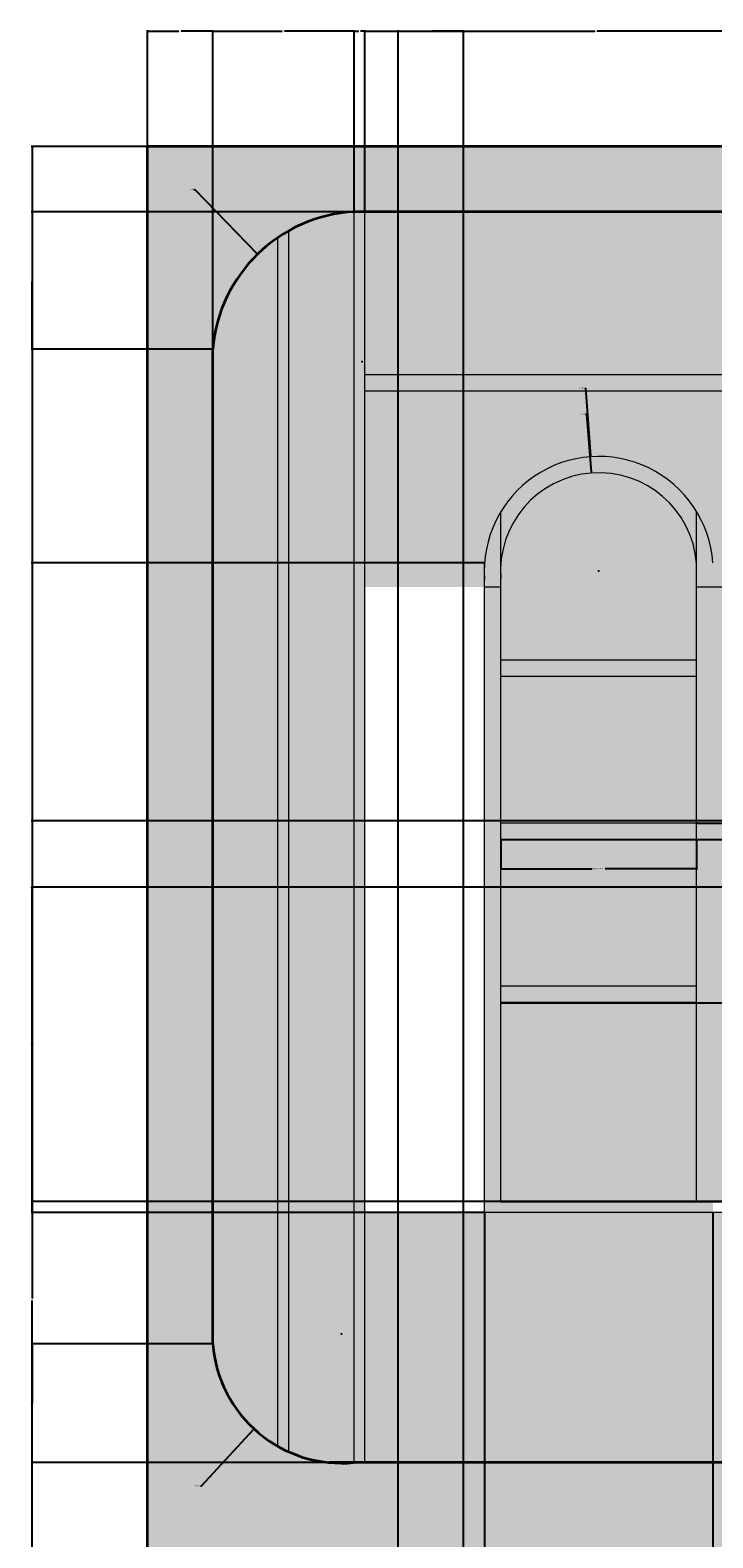
# Model space of a CAD drawing. Units: inches. Extents: x 2051 to 2334, y 814 to 1281.
# Tile 3 of 4: x 2051 to 2177, y 1003 to 1281. Entities that reach past the tile are written whole.
import ezdxf

# ---------------------------------------------------------------- set-up
doc = ezdxf.new("R2010")
doc.units = ezdxf.units.IN
for name, color, linetype, lineweight in [('A-ANNO-DIMS', 2, 'Continuous', 18), ('A-ELEV-FRAM', 7, 'Continuous', 35), ('A-ELEV-TRIM', 7, 'Continuous', 18), ('A-ELEV-TRIM-PATT', 7, 'Continuous', 13), ('A-GLAZ', 4, 'Continuous', 18), ('A-GLAZ-PATT', 4, 'Continuous', 13), ('A-ROOF', 7, 'Continuous', 35)]:
    doc.layers.add(name, color=color, linetype=linetype, lineweight=lineweight)
doc.layers.add('A-ELEV-FRAM-PATT', color=251, linetype='Continuous', lineweight=13, true_color=0x636466)
doc.layers.add('A-WALL-PATT', color=9, linetype='Continuous', lineweight=13, true_color=0xc7c8ca)
doc.styles.get("Standard").update_dxf_attribs({"font": 'arial.ttf'})
doc.dimstyles.get("Standard").update_dxf_attribs({"dimtxt": 0.18, "dimasz": 0.18, "dimexe": 0.18, "dimexo": 0.0625, "dimgap": 0.09, "dimtad": 0, "dimtih": 1, "dimtoh": 1, "dimdec": 4, "dimzin": 0, "dimdsep": 46, "dimtxsty": 'Standard', "dimcen": 0.09, "dimadec": 0, "dimazin": 0, "dimtfac": 1, "dimtdec": 4, "dimtofl": 0, "dimtmove": 0, "dimatfit": 3, "dimfxl": 1, "dimtolj": 1, "dimtzin": 0, "dimarcsym": 0})

# ---------------------------------------------------------------- blocks, each defined once
blk = doc.blocks.new('ARCH-LIGHT-TRANSOM-36X3')
for p, q in [((36, 3), (0, 3)), ((36, 0), (0, 0))]:
    blk.add_line(p, q)
blk = doc.blocks.new('*D5')
at = {"layer": 'A-ANNO-DIMS', "color": 0, "lineweight": -2, "transparency": 16777216}
for p, q in [((2137.93, 1131.75), (2137.93, 1126.23)), ((2173.93, 1131.75), (2173.93, 1126.23)), ((2138.11, 1126.41), (2154.73, 1126.41)), ((2173.75, 1126.41), (2157.12, 1126.41))]:
    blk.add_line(p, q, dxfattribs=at)
at = {"layer": 'A-ANNO-DIMS', "color": 0, "transparency": 16777216}
for points in [[(2138.11, 1126.44), (2138.11, 1126.38), (2137.93, 1126.41)], [(2173.75, 1126.44), (2173.75, 1126.38), (2173.93, 1126.41)]]:
    blk.add_solid(points, dxfattribs=at)
at = {"layer": 'Defpoints', "color": 0, "transparency": 16777216}
for p in [(2137.93, 1131.81), (2173.93, 1131.81), (2173.93, 1126.41)]:
    blk.add_point(p, dxfattribs=at)
at = {"layer": 'A-ANNO-DIMS', "color": 0, "transparency": 16777216, "insert": (2155.93, 1126.41), "char_height": 0.18, "attachment_point": 5}
blk.add_mtext('\\A1;TRANSOM 36 TYP.', dxfattribs=at)
blk = doc.blocks.new('*D6')
at = {"layer": 'A-ANNO-DIMS', "color": 0, "lineweight": -2, "transparency": 16777216}
for p, q in [((2173.99, 1134.81), (2179.51, 1134.81)), ((2179.33, 1134.63), (2179.33, 1133.5)), ((2173.99, 1131.81), (2179.51, 1131.81)), ((2179.33, 1131.99), (2179.33, 1133.13))]:
    blk.add_line(p, q, dxfattribs=at)
at = {"layer": 'A-ANNO-DIMS', "color": 0, "transparency": 16777216}
for points in [[(2179.3, 1134.63), (2179.36, 1134.63), (2179.33, 1134.81)], [(2179.3, 1131.99), (2179.36, 1131.99), (2179.33, 1131.81)]]:
    blk.add_solid(points, dxfattribs=at)
at = {"layer": 'Defpoints', "color": 0, "transparency": 16777216}
for p in [(2173.93, 1134.81), (2179.33, 1134.81), (2173.93, 1131.81)]:
    blk.add_point(p, dxfattribs=at)
at = {"layer": 'A-ANNO-DIMS', "color": 0, "transparency": 16777216, "insert": (2179.33, 1133.31), "char_height": 0.18, "attachment_point": 5}
blk.add_mtext('\\A1;3 TYP.', dxfattribs=at)
blk = doc.blocks.new('*D8')
at = {"layer": 'A-ANNO-DIMS', "color": 0, "lineweight": -2, "transparency": 16777216}
for p, q in [((2072.87, 1259.24), (2051.53, 1259.24)), ((2051.71, 1259.06), (2051.71, 1047.42)), ((2051.71, 835.42), (2051.71, 1047.06)), ((2072.87, 835.24), (2051.53, 835.24))]:
    blk.add_line(p, q, dxfattribs=at)
at = {"layer": 'A-ANNO-DIMS', "color": 0, "transparency": 16777216}
for points in [[(2051.68, 1259.06), (2051.74, 1259.06), (2051.71, 1259.24)], [(2051.68, 835.42), (2051.74, 835.42), (2051.71, 835.24)]]:
    blk.add_solid(points, dxfattribs=at)
at = {"layer": 'Defpoints', "color": 0, "transparency": 16777216}
for p in [(2051.71, 1259.24), (2072.93, 1259.24), (2072.93, 835.24)]:
    blk.add_point(p, dxfattribs=at)
at = {"layer": 'A-ANNO-DIMS', "color": 0, "transparency": 16777216, "insert": (2051.71, 1047.24), "char_height": 0.18, "attachment_point": 5}
blk.add_mtext('\\A1;424', dxfattribs=at)
blk = doc.blocks.new('*D16')
at = {"layer": 'A-ANNO-DIMS', "color": 0, "lineweight": -2, "transparency": 16777216}
for p, q in [((2072.93, 1259.31), (2072.93, 1280.64)), ((2073.11, 1280.46), (2078.72, 1280.46)), ((2084.75, 1280.46), (2079.14, 1280.46)), ((2084.93, 1222.02), (2084.93, 1280.64))]:
    blk.add_line(p, q, dxfattribs=at)
at = {"layer": 'A-ANNO-DIMS', "color": 0, "transparency": 16777216}
for points in [[(2073.11, 1280.49), (2073.11, 1280.43), (2072.93, 1280.46)], [(2084.75, 1280.49), (2084.75, 1280.43), (2084.93, 1280.46)]]:
    blk.add_solid(points, dxfattribs=at)
at = {"layer": 'Defpoints', "color": 0, "transparency": 16777216}
for p in [(2084.93, 1280.46), (2072.93, 1259.24), (2084.93, 1221.95)]:
    blk.add_point(p, dxfattribs=at)
at = {"layer": 'A-ANNO-DIMS', "color": 0, "transparency": 16777216, "insert": (2078.93, 1280.46), "char_height": 0.18, "attachment_point": 5}
blk.add_mtext('\\A1;12', dxfattribs=at)
blk = doc.blocks.new('*D17')
at = {"layer": 'A-ANNO-DIMS', "color": 0, "lineweight": -2, "transparency": 16777216}
for p, q in [((2084.93, 1222.02), (2084.93, 1280.64)), ((2085.11, 1280.46), (2097.71, 1280.46)), ((2110.75, 1280.46), (2098.15, 1280.46)), ((2110.93, 1247.31), (2110.93, 1280.64))]:
    blk.add_line(p, q, dxfattribs=at)
at = {"layer": 'A-ANNO-DIMS', "color": 0, "transparency": 16777216}
for points in [[(2085.11, 1280.49), (2085.11, 1280.43), (2084.93, 1280.46)], [(2110.75, 1280.49), (2110.75, 1280.43), (2110.93, 1280.46)]]:
    blk.add_solid(points, dxfattribs=at)
at = {"layer": 'Defpoints', "color": 0, "transparency": 16777216}
for p in [(2110.93, 1280.46), (2110.93, 1247.24), (2084.93, 1221.95)]:
    blk.add_point(p, dxfattribs=at)
at = {"layer": 'A-ANNO-DIMS', "color": 0, "transparency": 16777216, "insert": (2097.93, 1280.46), "char_height": 0.18, "attachment_point": 5}
blk.add_mtext('\\A1;26', dxfattribs=at)
blk = doc.blocks.new('*D18')
at = {"layer": 'A-ANNO-DIMS', "color": 0, "lineweight": -2, "transparency": 16777216}
for p, q in [((2110.93, 1247.31), (2110.93, 1280.64)), ((2111.11, 1280.46), (2111.78, 1280.46)), ((2112.75, 1280.46), (2112.08, 1280.46)), ((2112.93, 1247.31), (2112.93, 1280.64))]:
    blk.add_line(p, q, dxfattribs=at)
at = {"layer": 'A-ANNO-DIMS', "color": 0, "transparency": 16777216}
for points in [[(2111.11, 1280.49), (2111.11, 1280.43), (2110.93, 1280.46)], [(2112.75, 1280.49), (2112.75, 1280.43), (2112.93, 1280.46)]]:
    blk.add_solid(points, dxfattribs=at)
at = {"layer": 'Defpoints', "color": 0, "transparency": 16777216}
for p in [(2112.93, 1280.46), (2110.93, 1247.24), (2112.93, 1247.24)]:
    blk.add_point(p, dxfattribs=at)
at = {"layer": 'A-ANNO-DIMS', "color": 0, "transparency": 16777216, "insert": (2111.93, 1280.46), "char_height": 0.18, "attachment_point": 5}
blk.add_mtext('\\A1;2', dxfattribs=at)
blk = doc.blocks.new('*D19')
at = {"layer": 'A-ANNO-DIMS', "color": 0, "lineweight": -2, "transparency": 16777216}
for p, q in [((2112.93, 1247.31), (2112.93, 1280.64)), ((2113.11, 1280.46), (2155.21, 1280.46)), ((2197.75, 1280.46), (2155.65, 1280.46)), ((2197.93, 1247.31), (2197.93, 1280.64))]:
    blk.add_line(p, q, dxfattribs=at)
at = {"layer": 'A-ANNO-DIMS', "color": 0, "transparency": 16777216}
for points in [[(2113.11, 1280.49), (2113.11, 1280.43), (2112.93, 1280.46)], [(2197.75, 1280.49), (2197.75, 1280.43), (2197.93, 1280.46)]]:
    blk.add_solid(points, dxfattribs=at)
at = {"layer": 'Defpoints', "color": 0, "transparency": 16777216}
for p in [(2197.93, 1280.46), (2112.93, 1247.24), (2197.93, 1247.24)]:
    blk.add_point(p, dxfattribs=at)
at = {"layer": 'A-ANNO-DIMS', "color": 0, "transparency": 16777216, "insert": (2155.43, 1280.46), "char_height": 0.18, "attachment_point": 5}
blk.add_mtext('\\A1;85', dxfattribs=at)
blk = doc.blocks.new('*D23')
at = {"layer": 'A-ANNO-DIMS', "color": 0, "lineweight": -2, "transparency": 16777216}
for p, q in [((2084.87, 1039.06), (2051.53, 1039.06)), ((2051.71, 1038.88), (2051.71, 1028.33)), ((2051.71, 1017.42), (2051.71, 1027.97)), ((2110.87, 1017.24), (2051.53, 1017.24))]:
    blk.add_line(p, q, dxfattribs=at)
at = {"layer": 'A-ANNO-DIMS', "color": 0, "transparency": 16777216}
for points in [[(2051.68, 1038.88), (2051.74, 1038.88), (2051.71, 1039.06)], [(2051.68, 1017.42), (2051.74, 1017.42), (2051.71, 1017.24)]]:
    blk.add_solid(points, dxfattribs=at)
at = {"layer": 'Defpoints', "color": 0, "transparency": 16777216}
for p in [(2084.93, 1039.06), (2051.71, 1017.24), (2110.93, 1017.24)]:
    blk.add_point(p, dxfattribs=at)
at = {"layer": 'A-ANNO-DIMS', "color": 0, "transparency": 16777216, "insert": (2051.71, 1028.15), "char_height": 0.18, "attachment_point": 5}
blk.add_mtext('\\A1;21.81', dxfattribs=at)
blk = doc.blocks.new('*D24')
at = {"layer": 'A-ANNO-DIMS', "color": 0, "lineweight": -2, "transparency": 16777216}
for p, q in [((2110.87, 1247.24), (2051.53, 1247.24)), ((2051.71, 1247.06), (2051.71, 1234.78)), ((2051.71, 1222.13), (2051.71, 1234.42)), ((2084.87, 1221.95), (2051.53, 1221.95))]:
    blk.add_line(p, q, dxfattribs=at)
at = {"layer": 'A-ANNO-DIMS', "color": 0, "transparency": 16777216}
for points in [[(2051.68, 1247.06), (2051.74, 1247.06), (2051.71, 1247.24)], [(2051.68, 1222.13), (2051.74, 1222.13), (2051.71, 1221.95)]]:
    blk.add_solid(points, dxfattribs=at)
at = {"layer": 'Defpoints', "color": 0, "transparency": 16777216}
for p in [(2051.71, 1247.24), (2110.93, 1247.24), (2084.93, 1221.95)]:
    blk.add_point(p, dxfattribs=at)
at = {"layer": 'A-ANNO-DIMS', "color": 0, "transparency": 16777216, "insert": (2051.71, 1234.6), "char_height": 0.18, "attachment_point": 5}
blk.add_mtext('\\A1;25.29', dxfattribs=at)
blk = doc.blocks.new('*D25')
at = {"layer": 'A-ANNO-DIMS', "color": 0, "lineweight": -2, "transparency": 16777216}
for p, q in [((2134.87, 1182.7), (2051.53, 1182.7)), ((2051.71, 1182.52), (2051.71, 1123.15)), ((2051.71, 1063.42), (2051.71, 1122.79)), ((2134.87, 1063.24), (2051.53, 1063.24))]:
    blk.add_line(p, q, dxfattribs=at)
at = {"layer": 'A-ANNO-DIMS', "color": 0, "transparency": 16777216}
for points in [[(2051.68, 1182.52), (2051.74, 1182.52), (2051.71, 1182.7)], [(2051.68, 1063.42), (2051.74, 1063.42), (2051.71, 1063.24)]]:
    blk.add_solid(points, dxfattribs=at)
at = {"layer": 'Defpoints', "color": 0, "transparency": 16777216}
for p in [(2051.71, 1182.7), (2134.93, 1182.7), (2134.93, 1063.24)]:
    blk.add_point(p, dxfattribs=at)
at = {"layer": 'A-ANNO-DIMS', "color": 0, "transparency": 16777216, "insert": (2051.71, 1122.97), "char_height": 0.18, "attachment_point": 5}
blk.add_mtext('\\A1;119.45', dxfattribs=at)
blk = doc.blocks.new('*D26')
at = {"layer": 'A-ANNO-DIMS', "color": 0, "lineweight": -2, "transparency": 16777216}
for p, q in [((2203.87, 1123.07), (2051.53, 1123.07)), ((2051.71, 1122.89), (2051.71, 1094.34)), ((2051.71, 1065.42), (2051.71, 1093.98)), ((2203.87, 1065.24), (2051.53, 1065.24))]:
    blk.add_line(p, q, dxfattribs=at)
at = {"layer": 'A-ANNO-DIMS', "color": 0, "transparency": 16777216}
for points in [[(2051.68, 1122.89), (2051.74, 1122.89), (2051.71, 1123.07)], [(2051.68, 1065.42), (2051.74, 1065.42), (2051.71, 1065.24)]]:
    blk.add_solid(points, dxfattribs=at)
at = {"layer": 'Defpoints', "color": 0, "transparency": 16777216}
for p in [(2051.71, 1123.07), (2203.93, 1123.07), (2203.93, 1065.24)]:
    blk.add_point(p, dxfattribs=at)
at = {"layer": 'A-ANNO-DIMS', "color": 0, "transparency": 16777216, "insert": (2051.71, 1094.16), "char_height": 0.18, "attachment_point": 5}
blk.add_mtext('\\A1;57.83', dxfattribs=at)
blk = doc.blocks.new('*D27')
at = {"layer": 'A-ANNO-DIMS', "color": 0, "lineweight": -2, "transparency": 16777216}
for p, q in [((2134.93, 1063.18), (2134.93, 813.85)), ((2176.93, 1063.18), (2176.93, 813.85)), ((2135.11, 814.03), (2155.71, 814.03)), ((2176.75, 814.03), (2156.15, 814.03))]:
    blk.add_line(p, q, dxfattribs=at)
at = {"layer": 'A-ANNO-DIMS', "color": 0, "transparency": 16777216}
for points in [[(2135.11, 814.06), (2135.11, 814), (2134.93, 814.03)], [(2176.75, 814.06), (2176.75, 814), (2176.93, 814.03)]]:
    blk.add_solid(points, dxfattribs=at)
at = {"layer": 'Defpoints', "color": 0, "transparency": 16777216}
for p in [(2134.93, 1063.24), (2176.93, 1063.24), (2176.93, 814.03)]:
    blk.add_point(p, dxfattribs=at)
at = {"layer": 'A-ANNO-DIMS', "color": 0, "transparency": 16777216, "insert": (2155.93, 814.03), "char_height": 0.18, "attachment_point": 5}
blk.add_mtext('\\A1;42', dxfattribs=at)
blk = doc.blocks.new('*D28')
at = {"layer": 'A-ANNO-DIMS', "color": 0, "lineweight": -2, "transparency": 16777216}
for p, q in [((2203.93, 1065.18), (2203.93, 813.85)), ((2176.93, 1063.18), (2176.93, 813.85)), ((2177.11, 814.03), (2190.21, 814.03)), ((2203.75, 814.03), (2190.65, 814.03))]:
    blk.add_line(p, q, dxfattribs=at)
at = {"layer": 'A-ANNO-DIMS', "color": 0, "transparency": 16777216}
for points in [[(2177.11, 814.06), (2177.11, 814), (2176.93, 814.03)], [(2203.75, 814.06), (2203.75, 814), (2203.93, 814.03)]]:
    blk.add_solid(points, dxfattribs=at)
at = {"layer": 'Defpoints', "color": 0, "transparency": 16777216}
for p in [(2203.93, 1065.24), (2176.93, 1063.24), (2203.93, 814.03)]:
    blk.add_point(p, dxfattribs=at)
at = {"layer": 'A-ANNO-DIMS', "color": 0, "transparency": 16777216, "insert": (2190.43, 814.03), "char_height": 0.18, "attachment_point": 5}
blk.add_mtext('\\A1;27', dxfattribs=at)
blk = doc.blocks.new('*D31')
at = {"layer": 'A-ANNO-DIMS', "color": 0, "lineweight": -2, "transparency": 16777216}
for p, q in [((2137.99, 1101.81), (2334.32, 1101.81)), ((2334.14, 1101.63), (2334.14, 1083.71)), ((2334.14, 1065.42), (2334.14, 1083.35)), ((2137.99, 1065.24), (2334.32, 1065.24))]:
    blk.add_line(p, q, dxfattribs=at)
at = {"layer": 'A-ANNO-DIMS', "color": 0, "transparency": 16777216}
for points in [[(2334.11, 1101.63), (2334.17, 1101.63), (2334.14, 1101.81)], [(2334.11, 1065.42), (2334.17, 1065.42), (2334.14, 1065.24)]]:
    blk.add_solid(points, dxfattribs=at)
at = {"layer": 'Defpoints', "color": 0, "transparency": 16777216}
for p in [(2137.93, 1101.81), (2334.14, 1101.81), (2137.93, 1065.24)]:
    blk.add_point(p, dxfattribs=at)
at = {"layer": 'A-ANNO-DIMS', "color": 0, "transparency": 16777216, "insert": (2334.14, 1083.53), "char_height": 0.18, "attachment_point": 5}
blk.add_mtext('\\A1;36.57', dxfattribs=at)
blk = doc.blocks.new('*D32')
at = {"layer": 'A-ANNO-DIMS', "color": 0, "lineweight": -2, "transparency": 16777216}
for p, q in [((2137.99, 1131.81), (2334.32, 1131.81)), ((2334.14, 1131.63), (2334.14, 1117)), ((2334.14, 1101.99), (2334.14, 1116.63)), ((2137.99, 1101.81), (2334.32, 1101.81))]:
    blk.add_line(p, q, dxfattribs=at)
at = {"layer": 'A-ANNO-DIMS', "color": 0, "transparency": 16777216}
for points in [[(2334.11, 1131.63), (2334.17, 1131.63), (2334.14, 1131.81)], [(2334.11, 1101.99), (2334.17, 1101.99), (2334.14, 1101.81)]]:
    blk.add_solid(points, dxfattribs=at)
at = {"layer": 'Defpoints', "color": 0, "transparency": 16777216}
for p in [(2137.93, 1131.81), (2334.14, 1131.81), (2137.93, 1101.81)]:
    blk.add_point(p, dxfattribs=at)
at = {"layer": 'A-ANNO-DIMS', "color": 0, "transparency": 16777216, "insert": (2334.14, 1116.81), "char_height": 0.18, "attachment_point": 5}
blk.add_mtext('\\A1;30', dxfattribs=at)
blk = doc.blocks.new('*D33')
at = {"layer": 'A-ANNO-DIMS', "color": 0, "lineweight": -2, "transparency": 16777216}
for p, q in [((2246.87, 1135.24), (2051.53, 1135.24)), ((2051.71, 1135.06), (2051.71, 1100.43)), ((2051.71, 1065.42), (2051.71, 1100.06)), ((2246.87, 1065.24), (2051.53, 1065.24))]:
    blk.add_line(p, q, dxfattribs=at)
at = {"layer": 'A-ANNO-DIMS', "color": 0, "transparency": 16777216}
for points in [[(2051.68, 1135.06), (2051.74, 1135.06), (2051.71, 1135.24)], [(2051.68, 1065.42), (2051.74, 1065.42), (2051.71, 1065.24)]]:
    blk.add_solid(points, dxfattribs=at)
at = {"layer": 'Defpoints', "color": 0, "transparency": 16777216}
for p in [(2051.71, 1135.24), (2246.93, 1135.24), (2246.93, 1065.24)]:
    blk.add_point(p, dxfattribs=at)
at = {"layer": 'A-ANNO-DIMS', "color": 0, "transparency": 16777216, "insert": (2051.71, 1100.24), "char_height": 0.18, "attachment_point": 5}
blk.add_mtext('\\A1;70', dxfattribs=at)
blk = doc.blocks.new('*D43')
at = {"layer": 'A-ANNO-DIMS', "color": 0, "lineweight": -2, "transparency": 16777216}
for p, q in [((2119.03, 944.45), (2119.03, 1280.64)), ((2119.21, 1280.46), (2124.82, 1280.46)), ((2130.85, 1280.46), (2125.24, 1280.46)), ((2131.03, 944.45), (2131.03, 1280.64))]:
    blk.add_line(p, q, dxfattribs=at)
at = {"layer": 'A-ANNO-DIMS', "color": 0, "transparency": 16777216}
for points in [[(2119.21, 1280.49), (2119.21, 1280.43), (2119.03, 1280.46)], [(2130.85, 1280.49), (2130.85, 1280.43), (2131.03, 1280.46)]]:
    blk.add_solid(points, dxfattribs=at)
at = {"layer": 'Defpoints', "color": 0, "transparency": 16777216}
for p in [(2131.03, 1280.46), (2119.03, 944.38), (2131.03, 944.38)]:
    blk.add_point(p, dxfattribs=at)
at = {"layer": 'A-ANNO-DIMS', "color": 0, "transparency": 16777216, "insert": (2125.03, 1280.46), "char_height": 0.18, "attachment_point": 5}
blk.add_mtext('\\A1;12', dxfattribs=at)
blk = doc.blocks.new('*D55')
at = {"layer": 'A-ANNO-DIMS', "color": 0, "lineweight": -2, "transparency": 16777216}
for p, q in [((2081.46, 1251.34), (2081.64, 1251.34)), ((2081.64, 1251.34), (2093.07, 1239.6)), ((2112.35, 1219.68), (2112.53, 1219.68)), ((2112.44, 1219.59), (2112.44, 1219.77))]:
    blk.add_line(p, q, dxfattribs=at)
at = {"layer": 'A-ANNO-DIMS', "color": 0, "transparency": 16777216}
blk.add_solid([(2093.09, 1239.62), (2093.04, 1239.58), (2093.19, 1239.47)], dxfattribs=at)
at = {"layer": 'Defpoints', "color": 0, "transparency": 16777216}
for p in [(2093.19, 1239.47), (2112.44, 1219.68)]:
    blk.add_point(p, dxfattribs=at)
at = {"layer": 'A-ANNO-DIMS', "color": 0, "transparency": 16777216, "insert": (2081.05, 1251.34), "char_height": 0.18, "attachment_point": 5}
blk.add_mtext('\\A1;R27.6', dxfattribs=at)
blk = doc.blocks.new('*D56')
at = {"layer": 'A-ANNO-DIMS', "color": 0, "lineweight": -2, "transparency": 16777216}
for p, q in [((2108.55, 1040.92), (2108.73, 1040.92)), ((2108.64, 1040.83), (2108.64, 1041.01)), ((2082.85, 1012.94), (2092.4, 1023.3)), ((2082.67, 1012.94), (2082.85, 1012.94))]:
    blk.add_line(p, q, dxfattribs=at)
at = {"layer": 'A-ANNO-DIMS', "color": 0, "transparency": 16777216}
blk.add_solid([(2092.38, 1023.32), (2092.42, 1023.28), (2092.52, 1023.43)], dxfattribs=at)
at = {"layer": 'Defpoints', "color": 0, "transparency": 16777216}
for p in [(2108.64, 1040.92), (2092.52, 1023.43)]:
    blk.add_point(p, dxfattribs=at)
at = {"layer": 'A-ANNO-DIMS', "color": 0, "transparency": 16777216, "insert": (2082.12, 1012.94), "char_height": 0.18, "attachment_point": 5}
blk.add_mtext('\\A1;R23.785', dxfattribs=at)
blk = doc.blocks.new('*D59')
at = {"layer": 'A-ANNO-DIMS', "color": 0, "lineweight": -2, "transparency": 16777216}
for p, q in [((2153.35, 1214.8), (2153.53, 1214.8)), ((2153.53, 1214.8), (2154.42, 1202.38)), ((2155.84, 1181.2), (2156.02, 1181.2)), ((2155.93, 1181.11), (2155.93, 1181.29))]:
    blk.add_line(p, q, dxfattribs=at)
at = {"layer": 'A-ANNO-DIMS', "color": 0, "transparency": 16777216}
blk.add_solid([(2154.45, 1202.38), (2154.39, 1202.38), (2154.43, 1202.2)], dxfattribs=at)
at = {"layer": 'Defpoints', "color": 0, "transparency": 16777216}
for p in [(2154.43, 1202.2), (2155.93, 1181.2)]:
    blk.add_point(p, dxfattribs=at)
at = {"layer": 'A-ANNO-DIMS', "color": 0, "transparency": 16777216, "insert": (2152.8, 1214.8), "char_height": 0.18, "attachment_point": 5}
blk.add_mtext('\\A1;R21.054', dxfattribs=at)
blk = doc.blocks.new('*D60')
at = {"layer": 'A-ANNO-DIMS', "color": 0, "lineweight": -2, "transparency": 16777216}
for p, q in [((2153.53, 1210), (2153.71, 1210)), ((2153.71, 1210), (2154.53, 1199.38)), ((2155.84, 1181.2), (2156.02, 1181.2)), ((2155.93, 1181.11), (2155.93, 1181.29))]:
    blk.add_line(p, q, dxfattribs=at)
at = {"layer": 'A-ANNO-DIMS', "color": 0, "transparency": 16777216}
blk.add_solid([(2154.56, 1199.38), (2154.5, 1199.38), (2154.54, 1199.2)], dxfattribs=at)
at = {"layer": 'Defpoints', "color": 0, "transparency": 16777216}
for p in [(2154.54, 1199.2), (2155.93, 1181.2)]:
    blk.add_point(p, dxfattribs=at)
at = {"layer": 'A-ANNO-DIMS', "color": 0, "transparency": 16777216, "insert": (2152.98, 1210), "char_height": 0.18, "attachment_point": 5}
blk.add_mtext('\\A1;R18.054', dxfattribs=at)

msp = doc.modelspace()

# ---------------------------------------------------------------- hatches: boundary and pattern name
at = {"layer": 'A-ELEV-FRAM-PATT'}
h = msp.add_hatch(color=256, dxfattribs=at)
h.dxf.hatch_style = 1
h.paths.add_polyline_path([(2312.9283, 1217.2439), (2303.9283, 1217.2439), (2303.9283, 1059.2439, -0.29083376), (2256.3338, 1017.2439), (2110.9283, 1017.2439, -0.41949346), (2084.9283, 1039.0559), (2084.9283, 1221.9535, -0.37464242), (2110.9283, 1247.2439), (2247.6639, 1247.2439), (2247.6639, 1259.2439), (2072.9283, 1259.2439), (2072.9283, 835.2439), (2084.9283, 835.2439), (2084.9283, 967.2832, -0.36016597), (2115.4224, 997.2439), (2312.9283, 997.2439)])
at = {"layer": 'A-ELEV-TRIM-PATT'}
h = msp.add_hatch(color=256, dxfattribs=at)
h.dxf.hatch_style = 1
h.paths.add_polyline_path([(2112.9283, 1247.2439), (2110.9283, 1247.2439), (2110.9283, 1017.2439), (2112.9283, 1017.2439)])
h = msp.add_hatch(color=256, dxfattribs=at)
h.dxf.hatch_style = 1
h.paths.add_polyline_path([(2098.9283, 1243.754, 0.02131102), (2096.9283, 1242.5167), (2096.9283, 1020.2168, 0.02356469), (2098.9283, 1019.2065)])
h.paths.add_polyline_path([(2303.9283, 1217.2439), (2112.9283, 1217.2439), (2112.9283, 1214.2439), (2303.9283, 1214.2439)])
h.paths.add_polyline_path([(2303.9283, 1178.2439), (2176.9283, 1178.2439), (2176.9283, 1175.2439), (2303.9283, 1175.2439)])
h.paths.add_polyline_path([(2176.9283, 1182.698, 0.9311192), (2134.9283, 1182.698), (2134.9283, 1063.2439), (2176.9283, 1063.2439)])
h.paths.add_polyline_path([(2173.9283, 1065.2439), (2137.9283, 1065.2439), (2137.9283, 1182.698), (2137.9372, 1182.698, -0.9229497), (2173.9283, 1182.5869)], flags=16)
h = msp.add_hatch(color=256, dxfattribs=at)
h.dxf.hatch_style = 1
h.paths.add_polyline_path([(2173.9283, 1104.8149), (2137.9283, 1104.8149), (2137.9283, 1101.8149), (2173.9283, 1101.8149)])
h.paths.add_polyline_path([(2173.9283, 1134.8149), (2137.9283, 1134.8149), (2137.9283, 1131.8149), (2173.9283, 1131.8149)])
h.paths.add_polyline_path([(2173.9283, 1164.8149), (2137.9283, 1164.8149), (2137.9283, 1161.8149), (2173.9283, 1161.8149)])
at = {"layer": 'A-GLAZ-PATT', "transparency": 33554595}
h = msp.add_hatch(color=256, dxfattribs=at)
h.dxf.hatch_style = 1
h.set_gradient(color1=(255, 255, 255), color2=(0, 255, 255), name='INVCURVED')
h.paths.add_polyline_path([(2303.9283, 1214.2439), (2112.9283, 1214.2439), (2112.9283, 1178.2439), (2134.9283, 1178.2439), (2134.9283, 1182.698, -0.9311192), (2176.9283, 1182.698), (2176.9283, 1178.2439), (2303.9283, 1178.2439)])
at = {"layer": 'A-GLAZ-PATT', "transparency": 33554597}
h = msp.add_hatch(color=256, dxfattribs=at)
h.dxf.hatch_style = 1
h.set_gradient(color1=(255, 255, 255), color2=(147, 149, 152), name='INVCYLINDER')
h.paths.add_polyline_path([(2137.9283, 1182.5869), (2137.9283, 1164.8149), (2173.9283, 1164.8149), (2173.9283, 1182.5869, 0.92581255)])
h = msp.add_hatch(color=256, dxfattribs=at)
h.dxf.hatch_style = 1
h.set_gradient(color1=(255, 255, 255), color2=(147, 149, 152), name='INVCYLINDER')
h.paths.add_polyline_path([(2173.9283, 1161.8149), (2137.9283, 1161.8149), (2137.9283, 1134.8149), (2173.9283, 1134.8149)])
h = msp.add_hatch(color=256, dxfattribs=at)
h.dxf.hatch_style = 1
h.set_gradient(color1=(255, 255, 255), color2=(147, 149, 152), name='INVCYLINDER')
h.paths.add_polyline_path([(2173.9283, 1131.8149), (2137.9283, 1131.8149), (2137.9283, 1104.8149), (2173.9283, 1104.8149)])
h = msp.add_hatch(color=256, dxfattribs=at)
h.dxf.hatch_style = 1
h.set_gradient(color1=(255, 255, 255), color2=(147, 149, 152), name='INVCYLINDER')
h.paths.add_polyline_path([(2173.9283, 1101.8149), (2137.9283, 1101.8149), (2137.9283, 1065.2439), (2173.9283, 1065.2439)])
at = {"layer": 'A-GLAZ-PATT', "transparency": 33554595}
h = msp.add_hatch(color=256, dxfattribs=at)
h.dxf.hatch_style = 1
h.set_gradient(color1=(255, 255, 255), color2=(0, 255, 255), name='INVCURVED')
h.paths.add_polyline_path([(2303.9283, 1059.2439), (2303.9283, 1063.2439), (2112.9283, 1063.2439), (2112.9283, 1017.2439), (2256.3338, 1017.2439, 0.29083376)])
at = {"layer": 'A-WALL-PATT'}
h = msp.add_hatch(color=256, dxfattribs=at)
h.dxf.hatch_style = 1
h.paths.add_polyline_path([(2188.9283, 910.0037, 0.33864929), (2153.1397, 937.3832), (2125.034, 937.3832), (2125.034, 859.2439), (2188.9283, 859.2439)])
h.paths.add_polyline_path([(2113.034, 937.3832), (2084.9283, 937.3832), (2084.9283, 859.2439), (2113.034, 859.2439)])
h.paths.add_polyline_path([(2312.9283, 859.2439), (2084.9283, 859.2439), (2084.9283, 835.2439), (2312.9283, 835.2439)])
h.paths.add_polyline_path([(2288.9283, 1123.0714), (2288.9283, 1065.2439), (2303.9283, 1065.2439), (2303.9283, 1175.2439), (2176.9283, 1175.2439), (2176.9283, 1065.2439), (2203.9283, 1065.2439), (2203.9283, 1123.0714, -0.93632991)])
h.paths.add_polyline_path([(2197.9283, 1247.2439), (2112.9283, 1247.2439), (2112.9283, 1217.2439), (2197.9283, 1217.2439)])
h.paths.add_polyline_path([(2110.9283, 1247.2439, 0.11468321), (2098.9283, 1243.754), (2098.9283, 1019.2065, 0.12996728), (2110.9283, 1017.2439)])
h.paths.add_polyline_path([(2096.9283, 1242.5167, 0.22673474), (2084.9283, 1221.9535), (2084.9283, 1039.0559, 0.24937907), (2096.9283, 1020.2168)])

# ---------------------------------------------------------------- linework, layer by layer
at = {"layer": 'A-ELEV-FRAM'}
for p, q in [((2072.9283, 835.2439), (2072.9283, 1259.2439)), ((2084.9283, 1039.0559), (2084.9283, 1221.9535)), ((2256.3338, 1017.2439), (2106.3513, 1017.2439))]:
    msp.add_line(p, q, dxfattribs=at)
for centre, radius, start, end in [((2112.436, 1219.684), 27.6011, 93.131256, 175.283581), ((2108.6398, 1040.918), 23.7845, 184.490521, 275.521444)]:
    msp.add_arc(centre, radius, start, end, dxfattribs=at)
at = {"layer": 'A-ELEV-TRIM'}
for p, q in [((2110.9283, 1017.2439), (2110.9283, 1247.2439)), ((2112.9283, 1017.2439), (2112.9283, 1247.2439)), ((2096.9283, 1020.2168), (2096.9283, 1242.5167)), ((2098.9283, 1019.2065), (2098.9283, 1243.754)), ((2312.9283, 1217.2439), (2112.9283, 1217.2439)), ((2303.9283, 1214.2439), (2112.9283, 1214.2439)), ((2137.9283, 1178.2439), (2134.9283, 1178.2439)), ((2303.9283, 1178.2439), (2173.9283, 1178.2439)), ((2303.9283, 1063.2439), (2134.9283, 1063.2439))]:
    msp.add_line(p, q, dxfattribs=at)
at = {"layer": 'A-GLAZ'}
for p, q in [((2137.9283, 1065.2439), (2137.9283, 1192.1181)), ((2173.9283, 1065.2439), (2173.9283, 1192.1181)), ((2134.9283, 1063.2439), (2134.9283, 1182.698)), ((2137.9372, 1182.698), (2137.9283, 1182.698)), ((2173.9283, 1065.2439), (2137.9283, 1065.2439))]:
    msp.add_line(p, q, dxfattribs=at)
for radius, start, end in [(21.0535, 4.085617, 184.085617), (18.0535, 4.412192, 184.412192)]:
    msp.add_arc((2155.9283, 1181.198), radius, start, end, dxfattribs=at)
at = {"layer": 'A-ROOF'}
for p, q in [((2247.6639, 1259.2439), (2072.9283, 1259.2439)), ((2247.6639, 1247.2439), (2110.9283, 1247.2439))]:
    msp.add_line(p, q, dxfattribs=at)

# ---------------------------------------------------------------- block references
at = {"layer": 'A-GLAZ'}
for p in [(2137.9283, 1161.8149), (2137.9283, 1131.8149), (2137.9283, 1101.8149)]:
    msp.add_blockref('ARCH-LIGHT-TRANSOM-36X3', p, dxfattribs=at)

# ---------------------------------------------------------------- dimensions: what is measured, and where the dimension line sits
at = {"layer": 'A-ANNO-DIMS'}
for base, p1, p2, picture, middle in [((2084.9283, 1280.4589), (2072.9283, 1259.2439), (2084.9283, 1221.9535), '*D16', (2078.9283, 1280.4589)), ((2110.9283, 1280.4589), (2084.9283, 1221.9535), (2110.9283, 1247.2439), '*D17', (2097.9283, 1280.4589)), ((2112.9283, 1280.4589), (2110.9283, 1247.2439), (2112.9283, 1247.2439), '*D18', (2111.9283, 1280.4589)), ((2197.9283, 1280.4589), (2112.9283, 1247.2439), (2197.9283, 1247.2439), '*D19', (2155.4283, 1280.4589)), ((2131.034, 1280.4589), (2119.034, 944.3832), (2131.034, 944.3832), '*D43', (2125.034, 1280.4589)), ((2203.9283, 814.0289), (2176.9283, 1063.2439), (2203.9283, 1065.2439), '*D28', (2190.4283, 814.0289)), ((2176.9283, 814.0289), (2134.9283, 1063.2439), (2176.9283, 1063.2439), '*D27', (2155.9283, 814.0289))]:
    dim = msp.add_linear_dim(base=base, p1=p1, p2=p2, dimstyle='Standard', override={"dimdec": 0, "dimlfac": 1, "dimrnd": 0, "dimzin": 0, "dimdsep": 46, "dimlunit": 2}, dxfattribs=at)
    dim.commit()
    dim.dimension.update_dxf_attribs({"geometry": picture, "text_midpoint": middle})
for base, p1, p2, override, picture, middle in [((2051.7133, 1259.2439), (2072.9283, 835.2439), (2072.9283, 1259.2439), {"dimdec": 0, "dimlfac": 1, "dimrnd": 0, "dimzin": 0, "dimdsep": 46, "dimlunit": 2}, '*D8', (2051.7133, 1047.2439)), ((2051.7133, 1247.2439), (2084.9283, 1221.9535), (2110.9283, 1247.2439), {"dimdec": 2, "dimlfac": 1, "dimrnd": 0, "dimzin": 0, "dimdsep": 46, "dimlunit": 2}, '*D24', (2051.7133, 1234.5987)), ((2051.7133, 1182.698), (2134.9283, 1063.2439), (2134.9283, 1182.698), {"dimdec": 2, "dimlfac": 1, "dimrnd": 0, "dimzin": 0, "dimdsep": 46, "dimlunit": 2}, '*D25', (2051.7133, 1122.9709)), ((2051.7133, 1135.2439), (2246.9283, 1065.2439), (2246.9283, 1135.2439), {"dimdec": 0, "dimlfac": 1, "dimrnd": 0, "dimzin": 0, "dimdsep": 46, "dimlunit": 2}, '*D33', (2051.7133, 1100.2439)), ((2334.1433, 1131.8149), (2137.9283, 1101.8149), (2137.9283, 1131.8149), {"dimdec": 0, "dimlfac": 1, "dimrnd": 0, "dimzin": 0, "dimdsep": 46, "dimlunit": 2}, '*D32', (2334.1433, 1116.8149)), ((2051.7133, 1123.0714), (2203.9283, 1065.2439), (2203.9283, 1123.0714), {"dimdec": 2, "dimlfac": 1, "dimrnd": 0, "dimzin": 0, "dimdsep": 46, "dimlunit": 2}, '*D26', (2051.7133, 1094.1576)), ((2334.1433, 1101.8149), (2137.9283, 1065.2439), (2137.9283, 1101.8149), {"dimdec": 2, "dimlfac": 1, "dimrnd": 0, "dimzin": 0, "dimdsep": 46, "dimlunit": 2}, '*D31', (2334.1433, 1083.5294)), ((2051.7133, 1017.2439), (2084.9283, 1039.0559), (2110.9283, 1017.2439), {"dimdec": 2, "dimlfac": 1, "dimrnd": 0, "dimzin": 0, "dimdsep": 46, "dimlunit": 2}, '*D23', (2051.7133, 1028.1499))]:
    dim = msp.add_linear_dim(base=base, p1=p1, p2=p2, angle=90, dimstyle='Standard', override=override, dxfattribs=at)
    dim.commit()
    dim.dimension.update_dxf_attribs({"geometry": picture, "text_midpoint": middle})
for center, mpoint, override, picture, middle in [((2112.436, 1219.684), (2093.1909, 1239.4691), {"dimdec": 1, "dimlfac": 1, "dimrnd": 0, "dimzin": 0, "dimdsep": 46, "dimlunit": 2}, '*D55', (2081.054, 1251.3401)), ((2155.9283, 1181.198), (2154.428, 1202.198), {"dimdec": 3, "dimlfac": 1, "dimrnd": 0, "dimzin": 0, "dimdsep": 46, "dimlunit": 2}, '*D59', (2152.7984, 1214.7979)), ((2155.928301, 1181.197976), (2154.539004, 1199.197943), {"dimdec": 3, "dimlfac": 1, "dimrnd": 0, "dimzin": 0, "dimdsep": 46, "dimlunit": 2}, '*D60', (2152.976033, 1209.997923)), ((2108.6398, 1040.91805), (2092.51958, 1023.42973), {"dimdec": 3, "dimlfac": 1, "dimrnd": 0, "dimzin": 0, "dimdsep": 46, "dimlunit": 2}, '*D56', (2082.11701, 1012.93674))]:
    dim = msp.add_radius_dim(center=center, mpoint=mpoint, dimstyle='Standard', override=override, dxfattribs=at)
    dim.commit()
    dim.dimension.update_dxf_attribs({"geometry": picture, "text_midpoint": middle, "dimtype": 164})
dim = msp.add_linear_dim(base=(2179.3283, 1134.8149), p1=(2173.9283, 1131.8149), p2=(2173.9283, 1134.8149), angle=90, text='<> TYP.', dimstyle='Standard', override={"dimdec": 0, "dimlfac": 1, "dimrnd": 0, "dimzin": 0, "dimdsep": 46, "dimlunit": 2}, dxfattribs=at)
dim.commit()
dim.dimension.update_dxf_attribs({"geometry": '*D6', "text_midpoint": (2179.3283, 1133.3149)})
dim = msp.add_linear_dim(base=(2173.9283, 1126.4149), p1=(2137.9283, 1131.8149), p2=(2173.9283, 1131.8149), text='TRANSOM <> TYP.', dimstyle='Standard', override={"dimdec": 0, "dimlfac": 1, "dimrnd": 0, "dimzin": 0, "dimdsep": 46, "dimlunit": 2}, dxfattribs=at)
dim.commit()
dim.dimension.update_dxf_attribs({"geometry": '*D5', "text_midpoint": (2155.9283, 1126.4149)})

doc.saveas('drawing.dxf')
